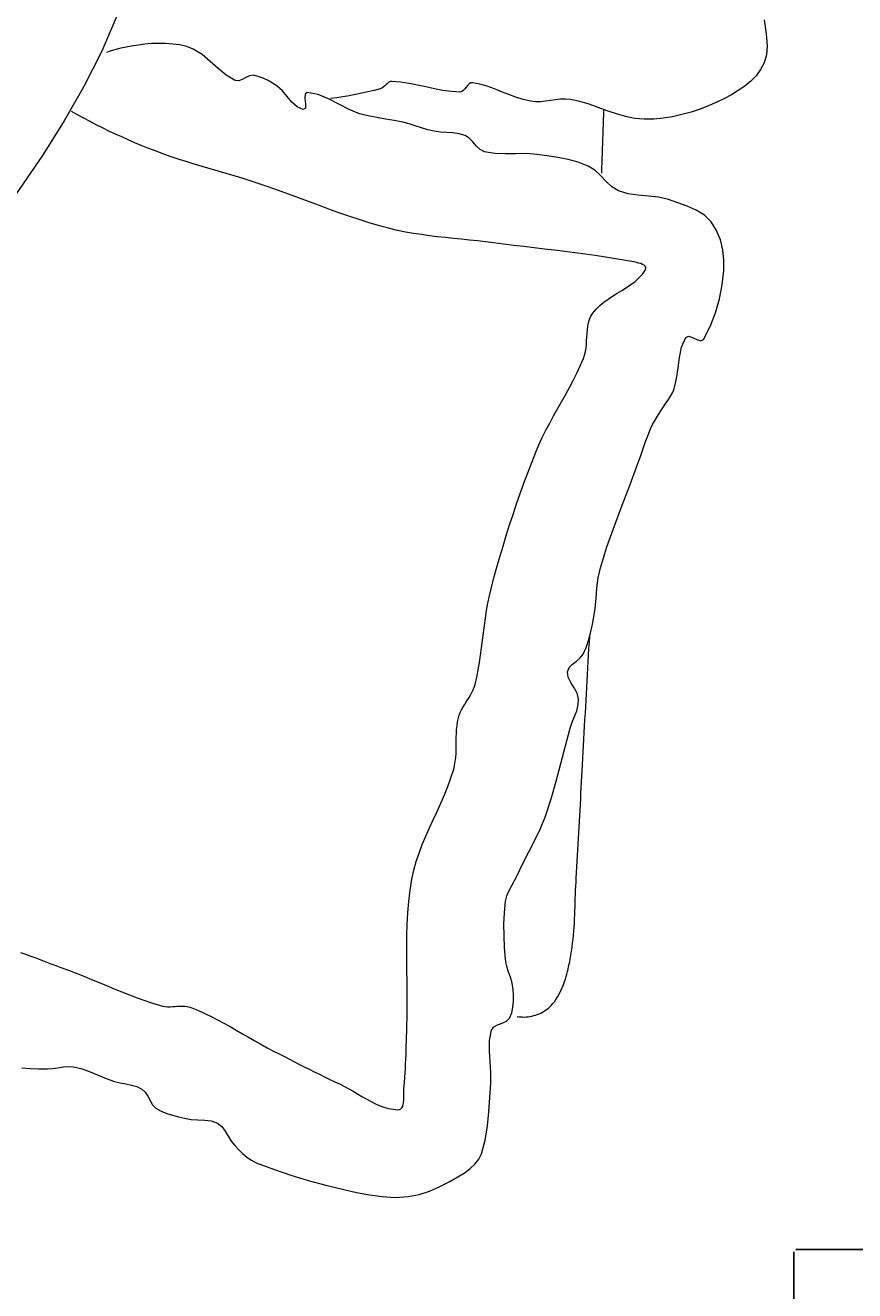
# Model space of a CAD drawing. Units: inches. Extents: x -15 to 423, y -713 to 71.
# Tile 21 of 24: x 340 to 364, y -173 to -137. Entities that reach past the tile are written whole.
import ezdxf

# ---------------------------------------------------------------- set-up
doc = ezdxf.new("R2010")
doc.units = ezdxf.units.IN
doc.header["$MEASUREMENT"] = 0
doc.layers.add('A-ANNO-DIMS', color=2, linetype='Continuous', lineweight=18)
doc.layers.add('A-FURN', color=9, linetype='Continuous', lineweight=13)
doc.styles.get("Standard").update_dxf_attribs({"font": 'arial.ttf'})
doc.dimstyles.get("Standard").update_dxf_attribs({"dimtxt": 0.18, "dimasz": 0.18, "dimexe": 0.18, "dimexo": 0.0625, "dimgap": 0.09, "dimtad": 0, "dimtih": 1, "dimtoh": 1, "dimdec": 0, "dimzin": 0, "dimdsep": 46, "dimlunit": 3, "dimtxsty": 'Standard', "dimcen": 0.09, "dimadec": 0, "dimazin": 0, "dimtfac": 1, "dimtdec": 0, "dimtofl": 0, "dimtmove": 0, "dimatfit": 3, "dimfxl": 1, "dimtolj": 1, "dimtzin": 0, "dimarcsym": 0})

# ---------------------------------------------------------------- blocks, each defined once
blk = doc.blocks.new('BED-DOUBLE')
for p, q in [((81.158, 34.884), (80.717, 33.859)), ((99.427, 34.751), (99.468, 34.498)), ((99.468, 34.498), (99.501, 34.248)), ((81.553, 34.002), (81.363, 33.968)), ((81.743, 34.034), (81.553, 34.002)), ((81.934, 34.06), (81.743, 34.034)), ((82.126, 34.077), (81.934, 34.06)), ((82.318, 34.081), (82.126, 34.077)), ((82.52, 34.075), (82.318, 34.081)), ((82.723, 34.063), (82.52, 34.075)), ((82.924, 34.037), (82.723, 34.063)), ((83.119, 33.992), (82.924, 34.037)), ((83.305, 33.921), (83.119, 33.992)), ((99.514, 34.001), (99.494, 33.761)), ((99.501, 34.248), (99.514, 34.001)), ((80.717, 33.859), (80.211, 32.862)), ((80.953, 33.862), (80.854, 33.825)), ((81.054, 33.894), (80.953, 33.862)), ((81.156, 33.923), (81.054, 33.894)), ((81.259, 33.948), (81.156, 33.923)), ((81.363, 33.968), (81.259, 33.948)), ((83.556, 33.766), (83.305, 33.921)), ((83.784, 33.574), (83.556, 33.766)), ((99.494, 33.761), (99.427, 33.528)), ((84.005, 33.372), (83.784, 33.574)), ((84.235, 33.184), (84.005, 33.372)), ((99.329, 33.34), (99.203, 33.169)), ((99.427, 33.528), (99.329, 33.34)), ((84.489, 33.037), (84.235, 33.184)), ((84.587, 33.027), (84.489, 33.037)), ((84.687, 33.064), (84.587, 33.027)), ((84.79, 33.12), (84.687, 33.064)), ((84.893, 33.168), (84.79, 33.12)), ((84.998, 33.18), (84.893, 33.168)), ((85.142, 33.148), (84.998, 33.18)), ((85.281, 33.097), (85.142, 33.148)), ((85.416, 33.031), (85.281, 33.097)), ((85.546, 32.954), (85.416, 33.031)), ((85.67, 32.872), (85.546, 32.954)), ((88.75, 32.919), (88.711, 32.883)), ((88.789, 32.953), (88.75, 32.919)), ((88.829, 32.982), (88.789, 32.953)), ((88.872, 33.001), (88.829, 32.982)), ((88.919, 33.007), (88.872, 33.001)), ((89.161, 32.986), (88.919, 33.007)), ((89.4, 32.95), (89.161, 32.986)), ((89.639, 32.903), (89.4, 32.95)), ((89.877, 32.851), (89.639, 32.903)), ((91.096, 32.937), (91.054, 32.895)), ((91.141, 32.965), (91.096, 32.937)), ((91.192, 32.971), (91.141, 32.965)), ((91.403, 32.931), (91.192, 32.971)), ((91.609, 32.871), (91.403, 32.931)), ((99.053, 33.014), (98.884, 32.874)), ((99.203, 33.169), (99.053, 33.014)), ((80.211, 32.862), (79.655, 31.89)), ((85.821, 32.738), (85.67, 32.872)), ((85.956, 32.578), (85.821, 32.738)), ((86.09, 32.42), (85.956, 32.578)), ((86.462, 32.647), (86.458, 32.521)), ((86.521, 32.696), (86.462, 32.647)), ((86.831, 32.634), (86.521, 32.696)), ((87.126, 32.514), (86.831, 32.634)), ((87.356, 32.547), (87.178, 32.524)), ((87.533, 32.573), (87.356, 32.547)), ((87.71, 32.603), (87.533, 32.573)), ((87.886, 32.636), (87.71, 32.603)), ((88.062, 32.672), (87.886, 32.636)), ((88.237, 32.712), (88.062, 32.672)), ((88.411, 32.755), (88.237, 32.712)), ((88.584, 32.801), (88.411, 32.755)), ((88.629, 32.82), (88.584, 32.801)), ((88.671, 32.849), (88.629, 32.82)), ((88.711, 32.883), (88.671, 32.849)), ((90.116, 32.799), (89.877, 32.851)), ((90.355, 32.755), (90.116, 32.799)), ((90.595, 32.722), (90.355, 32.755)), ((90.836, 32.707), (90.595, 32.722)), ((90.888, 32.719), (90.836, 32.707)), ((90.933, 32.75), (90.888, 32.719)), ((90.975, 32.795), (90.933, 32.75)), ((91.015, 32.845), (90.975, 32.795)), ((91.054, 32.895), (91.015, 32.845)), ((91.812, 32.797), (91.609, 32.871)), ((92.013, 32.716), (91.812, 32.797)), ((92.214, 32.634), (92.013, 32.716)), ((92.417, 32.558), (92.214, 32.634)), ((92.622, 32.492), (92.417, 32.558)), ((98.509, 32.632), (98.313, 32.528)), ((98.701, 32.747), (98.509, 32.632)), ((98.884, 32.874), (98.701, 32.747)), ((86.237, 32.289), (86.09, 32.42)), ((86.412, 32.213), (86.237, 32.289)), ((86.47, 32.251), (86.412, 32.213)), ((86.458, 32.521), (86.473, 32.372)), ((86.473, 32.372), (86.47, 32.251)), ((87.415, 32.365), (87.126, 32.514)), ((87.705, 32.216), (87.415, 32.365)), ((88.003, 32.096), (87.705, 32.216)), ((92.831, 32.445), (92.622, 32.492)), ((92.971, 32.431), (92.831, 32.445)), ((93.112, 32.434), (92.971, 32.431)), ((93.253, 32.448), (93.112, 32.434)), ((93.395, 32.468), (93.253, 32.448)), ((93.537, 32.488), (93.395, 32.468)), ((93.679, 32.503), (93.537, 32.488)), ((93.82, 32.507), (93.679, 32.503)), ((93.96, 32.495), (93.82, 32.507)), ((94.224, 32.44), (93.96, 32.495)), ((94.484, 32.363), (94.224, 32.44)), ((94.742, 32.273), (94.484, 32.363)), ((94.999, 32.179), (94.742, 32.273)), ((94.902, 32.129), (94.905, 32.22)), ((97.622, 32.227), (97.367, 32.141)), ((97.873, 32.324), (97.622, 32.227)), ((98.117, 32.433), (97.873, 32.324)), ((98.313, 32.528), (98.117, 32.433)), ((79.655, 31.89), (79.064, 30.944)), ((80.036, 32.061), (79.861, 32.158)), ((80.211, 31.966), (80.036, 32.061)), ((80.387, 31.873), (80.211, 31.966)), ((80.565, 31.782), (80.387, 31.873)), ((88.243, 32.032), (88.003, 32.096)), ((88.487, 31.984), (88.243, 32.032)), ((88.732, 31.944), (88.487, 31.984)), ((88.978, 31.903), (88.732, 31.944)), ((89.222, 31.853), (88.978, 31.903)), ((89.4, 31.805), (89.222, 31.853)), ((94.89, 31.768), (94.893, 31.858)), ((94.893, 31.858), (94.896, 31.949)), ((94.896, 31.949), (94.899, 32.039)), ((94.899, 32.039), (94.902, 32.129)), ((95.257, 32.09), (94.999, 32.179)), ((95.516, 32.015), (95.257, 32.09)), ((95.778, 31.962), (95.516, 32.015)), ((96.045, 31.939), (95.778, 31.962)), ((96.312, 31.945), (96.045, 31.939)), ((96.578, 31.969), (96.312, 31.945)), ((96.843, 32.011), (96.578, 31.969)), ((97.107, 32.069), (96.843, 32.011)), ((97.367, 32.141), (97.107, 32.069)), ((80.743, 31.692), (80.565, 31.782)), ((80.923, 31.605), (80.743, 31.692)), ((81.104, 31.52), (80.923, 31.605)), ((81.285, 31.437), (81.104, 31.52)), ((89.577, 31.751), (89.4, 31.805)), ((89.753, 31.695), (89.577, 31.751)), ((89.93, 31.642), (89.753, 31.695)), ((90.109, 31.598), (89.93, 31.642)), ((90.284, 31.573), (90.109, 31.598)), ((90.462, 31.562), (90.284, 31.573)), ((90.639, 31.551), (90.462, 31.562)), ((90.814, 31.528), (90.639, 31.551)), ((90.981, 31.479), (90.814, 31.528)), ((91.101, 31.403), (90.981, 31.479)), ((94.877, 31.407), (94.88, 31.497)), ((94.88, 31.497), (94.883, 31.587)), ((94.883, 31.587), (94.886, 31.678)), ((94.886, 31.678), (94.89, 31.768)), ((81.468, 31.355), (81.285, 31.437)), ((81.651, 31.276), (81.468, 31.355)), ((81.835, 31.199), (81.651, 31.276)), ((82.02, 31.124), (81.835, 31.199)), ((82.205, 31.052), (82.02, 31.124)), ((91.205, 31.296), (91.101, 31.403)), ((91.303, 31.181), (91.205, 31.296)), ((91.408, 31.082), (91.303, 31.181)), ((94.864, 31.046), (94.867, 31.136)), ((94.867, 31.136), (94.871, 31.226)), ((94.871, 31.226), (94.874, 31.317)), ((94.874, 31.317), (94.877, 31.407)), ((79.064, 30.944), (77.93, 29.295)), ((82.427, 30.969), (82.205, 31.052)), ((82.65, 30.89), (82.427, 30.969)), ((82.874, 30.815), (82.65, 30.89)), ((83.099, 30.743), (82.874, 30.815)), ((91.533, 31.019), (91.408, 31.082)), ((91.823, 30.969), (91.533, 31.019)), ((92.118, 30.958), (91.823, 30.969)), ((92.416, 30.963), (92.118, 30.958)), ((92.714, 30.966), (92.416, 30.963)), ((93.009, 30.944), (92.714, 30.966)), ((93.304, 30.904), (93.009, 30.944)), ((93.601, 30.858), (93.304, 30.904)), ((93.894, 30.8), (93.601, 30.858)), ((94.181, 30.722), (93.894, 30.8)), ((94.852, 30.684), (94.855, 30.775)), ((94.855, 30.775), (94.858, 30.865)), ((94.858, 30.865), (94.861, 30.955)), ((94.861, 30.955), (94.864, 31.046)), ((83.325, 30.673), (83.099, 30.743)), ((83.552, 30.605), (83.325, 30.673)), ((83.779, 30.538), (83.552, 30.605)), ((84.006, 30.471), (83.779, 30.538)), ((84.233, 30.404), (84.006, 30.471)), ((84.46, 30.337), (84.233, 30.404)), ((94.458, 30.617), (94.181, 30.722)), ((94.644, 30.5), (94.458, 30.617)), ((94.808, 30.347), (94.644, 30.5)), ((94.842, 30.414), (94.845, 30.504)), ((94.845, 30.504), (94.848, 30.594)), ((94.848, 30.594), (94.852, 30.684)), ((84.686, 30.269), (84.46, 30.337)), ((84.912, 30.198), (84.686, 30.269)), ((85.137, 30.125), (84.912, 30.198)), ((85.424, 30.028), (85.137, 30.125)), ((94.964, 30.181), (94.808, 30.347)), ((95.128, 30.029), (94.964, 30.181)), ((85.709, 29.927), (85.424, 30.028)), ((85.993, 29.823), (85.709, 29.927)), ((86.277, 29.718), (85.993, 29.823)), ((86.561, 29.612), (86.277, 29.718)), ((95.316, 29.916), (95.128, 30.029)), ((95.589, 29.834), (95.316, 29.916)), ((95.873, 29.793), (95.589, 29.834)), ((96.162, 29.768), (95.873, 29.793)), ((96.45, 29.735), (96.162, 29.768)), ((96.728, 29.668), (96.45, 29.735)), ((86.845, 29.506), (86.561, 29.612)), ((87.129, 29.401), (86.845, 29.506)), ((87.414, 29.298), (87.129, 29.401)), ((96.993, 29.581), (96.728, 29.668)), ((97.26, 29.486), (96.993, 29.581)), ((97.515, 29.372), (97.26, 29.486)), ((97.746, 29.225), (97.515, 29.372)), ((87.699, 29.198), (87.414, 29.298)), ((87.986, 29.102), (87.699, 29.198)), ((88.275, 29.012), (87.986, 29.102)), ((88.565, 28.927), (88.275, 29.012)), ((97.937, 29.036), (97.746, 29.225)), ((98.089, 28.796), (97.937, 29.036)), ((88.857, 28.849), (88.565, 28.927)), ((89.078, 28.797), (88.857, 28.849)), ((89.3, 28.752), (89.078, 28.797)), ((89.523, 28.712), (89.3, 28.752)), ((89.748, 28.678), (89.523, 28.712)), ((89.973, 28.647), (89.748, 28.678)), ((90.198, 28.62), (89.973, 28.647)), ((90.425, 28.595), (90.198, 28.62)), ((98.197, 28.529), (98.089, 28.796)), ((90.651, 28.572), (90.425, 28.595)), ((90.878, 28.549), (90.651, 28.572)), ((91.104, 28.526), (90.878, 28.549)), ((91.33, 28.502), (91.104, 28.526)), ((91.556, 28.476), (91.33, 28.502)), ((91.782, 28.447), (91.556, 28.476)), ((92.069, 28.41), (91.782, 28.447)), ((92.357, 28.373), (92.069, 28.41)), ((92.645, 28.338), (92.357, 28.373)), ((92.934, 28.304), (92.645, 28.338)), ((93.222, 28.269), (92.934, 28.304)), ((93.51, 28.235), (93.222, 28.269)), ((98.265, 28.245), (98.197, 28.529)), ((93.798, 28.2), (93.51, 28.235)), ((94.086, 28.163), (93.798, 28.2)), ((94.374, 28.125), (94.086, 28.163)), ((94.661, 28.085), (94.374, 28.125)), ((94.948, 28.043), (94.661, 28.085)), ((95.235, 27.997), (94.948, 28.043)), ((95.52, 27.948), (95.235, 27.997)), ((95.572, 27.94), (95.52, 27.948)), ((95.63, 27.93), (95.572, 27.94)), ((95.692, 27.919), (95.63, 27.93)), ((95.757, 27.907), (95.692, 27.919)), ((95.823, 27.892), (95.757, 27.907)), ((95.886, 27.876), (95.823, 27.892)), ((98.296, 27.954), (98.265, 28.245)), ((98.293, 27.667), (98.296, 27.954)), ((95.945, 27.858), (95.886, 27.876)), ((95.893, 27.455), (95.992, 27.563)), ((95.997, 27.836), (95.945, 27.858)), ((95.992, 27.563), (96.078, 27.682)), ((96.04, 27.812), (95.997, 27.836)), ((96.072, 27.785), (96.04, 27.812)), ((96.09, 27.755), (96.072, 27.785)), ((96.078, 27.682), (96.093, 27.72)), ((96.093, 27.72), (96.09, 27.755)), ((98.248, 27.261), (98.293, 27.667)), ((95.41, 27.101), (95.539, 27.183)), ((95.539, 27.183), (95.664, 27.267)), ((95.664, 27.267), (95.783, 27.357)), ((95.783, 27.357), (95.893, 27.455)), ((98.169, 26.859), (98.248, 27.261)), ((94.9, 26.77), (95.022, 26.858)), ((95.022, 26.858), (95.149, 26.941)), ((95.149, 26.941), (95.279, 27.022)), ((95.279, 27.022), (95.41, 27.101)), ((98.054, 26.464), (98.169, 26.859)), ((94.59, 26.455), (94.682, 26.57)), ((94.682, 26.57), (94.786, 26.674)), ((94.786, 26.674), (94.9, 26.77)), ((97.904, 26.082), (98.054, 26.464)), ((94.453, 26.088), (94.473, 26.186)), ((94.473, 26.186), (94.501, 26.28)), ((94.501, 26.28), (94.539, 26.37)), ((94.539, 26.37), (94.59, 26.455)), ((94.417, 25.678), (94.423, 25.782)), ((94.423, 25.782), (94.43, 25.886)), ((94.43, 25.886), (94.439, 25.988)), ((94.439, 25.988), (94.453, 26.088)), ((97.1, 25.5), (97.217, 25.769)), ((97.217, 25.769), (97.294, 25.805)), ((97.294, 25.805), (97.407, 25.772)), ((97.407, 25.772), (97.532, 25.714)), ((97.721, 25.718), (97.904, 26.082)), ((94.382, 25.372), (94.399, 25.472)), ((94.399, 25.472), (94.41, 25.575)), ((94.41, 25.575), (94.417, 25.678)), ((97.037, 25.21), (97.1, 25.5)), ((97.532, 25.714), (97.645, 25.681)), ((97.645, 25.681), (97.721, 25.718)), ((94.235, 24.969), (94.326, 25.179)), ((94.326, 25.179), (94.359, 25.273)), ((94.359, 25.273), (94.382, 25.372)), ((96.999, 24.911), (97.037, 25.21)), ((94.035, 24.558), (94.138, 24.762)), ((94.138, 24.762), (94.235, 24.969)), ((96.959, 24.61), (96.999, 24.911)), ((93.818, 24.155), (93.928, 24.356)), ((93.928, 24.356), (94.035, 24.558)), ((96.841, 24.205), (96.89, 24.32)), ((96.89, 24.32), (96.959, 24.61)), ((93.706, 23.955), (93.818, 24.155)), ((96.634, 23.889), (96.707, 23.993)), ((96.707, 23.993), (96.778, 24.097)), ((96.778, 24.097), (96.841, 24.205)), ((93.482, 23.555), (93.593, 23.755)), ((93.593, 23.755), (93.706, 23.955)), ((96.421, 23.549), (96.494, 23.666)), ((96.494, 23.666), (96.566, 23.783)), ((96.566, 23.783), (96.634, 23.889)), ((93.265, 23.152), (93.372, 23.354)), ((93.372, 23.354), (93.482, 23.555)), ((96.221, 23.189), (96.281, 23.312)), ((96.281, 23.312), (96.349, 23.432)), ((96.349, 23.432), (96.421, 23.549)), ((93.068, 22.74), (93.164, 22.947)), ((93.164, 22.947), (93.265, 23.152)), ((96.069, 22.8), (96.141, 22.996)), ((96.141, 22.996), (96.221, 23.189)), ((92.864, 22.239), (92.979, 22.53)), ((92.979, 22.53), (93.068, 22.74)), ((95.935, 22.404), (96.002, 22.602)), ((96.002, 22.602), (96.069, 22.8)), ((92.753, 21.948), (92.864, 22.239)), ((95.648, 21.619), (95.867, 22.207)), ((95.867, 22.207), (95.935, 22.404)), ((92.644, 21.655), (92.753, 21.948)), ((92.539, 21.361), (92.644, 21.655)), ((95.422, 21.034), (95.648, 21.619)), ((92.436, 21.066), (92.539, 21.361)), ((92.24, 20.473), (92.337, 20.77)), ((92.337, 20.77), (92.436, 21.066)), ((95.2, 20.447), (95.422, 21.034)), ((92.146, 20.175), (92.24, 20.473)), ((94.99, 19.857), (95.2, 20.447)), ((92.055, 19.876), (92.146, 20.175)), ((91.967, 19.576), (92.055, 19.876)), ((94.804, 19.259), (94.99, 19.857)), ((91.882, 19.276), (91.967, 19.576)), ((91.719, 18.673), (91.799, 18.975)), ((91.799, 18.975), (91.882, 19.276)), ((94.707, 18.69), (94.742, 18.977)), ((94.742, 18.977), (94.804, 19.259)), ((91.669, 18.468), (91.719, 18.673)), ((94.683, 18.401), (94.707, 18.69)), ((91.59, 18.053), (91.627, 18.261)), ((91.627, 18.261), (91.669, 18.468)), ((94.657, 18.111), (94.683, 18.401)), ((91.558, 17.844), (91.59, 18.053)), ((94.613, 17.825), (94.657, 18.111)), ((91.502, 17.424), (91.529, 17.634)), ((91.529, 17.634), (91.558, 17.844)), ((94.524, 17.415), (94.571, 17.62)), ((94.571, 17.62), (94.613, 17.825)), ((91.449, 17.004), (91.476, 17.214)), ((91.476, 17.214), (91.502, 17.424)), ((94.4, 17.014), (94.468, 17.212)), ((94.468, 17.212), (94.524, 17.415)), ((94.494, 17.16), (94.504, 17.342)), ((91.421, 16.794), (91.449, 17.004)), ((94.236, 16.716), (94.317, 16.822)), ((94.317, 16.822), (94.4, 17.014)), ((94.473, 16.795), (94.483, 16.977)), ((94.483, 16.977), (94.494, 17.16)), ((91.353, 16.376), (91.389, 16.585)), ((91.389, 16.585), (91.421, 16.794)), ((93.922, 16.444), (94.013, 16.539)), ((94.013, 16.539), (94.126, 16.626)), ((94.126, 16.626), (94.236, 16.716)), ((94.452, 16.43), (94.463, 16.612)), ((94.463, 16.612), (94.473, 16.795)), ((91.264, 15.963), (91.312, 16.169)), ((91.312, 16.169), (91.353, 16.376)), ((93.877, 16.327), (93.922, 16.444)), ((93.898, 16.169), (93.877, 16.327)), ((93.971, 16.019), (93.898, 16.169)), ((94.432, 16.065), (94.442, 16.248)), ((94.442, 16.248), (94.452, 16.43)), ((91.137, 15.668), (91.176, 15.739)), ((91.176, 15.739), (91.211, 15.812)), ((91.211, 15.812), (91.241, 15.886)), ((91.241, 15.886), (91.264, 15.963)), ((94.065, 15.871), (93.971, 16.019)), ((94.149, 15.721), (94.065, 15.871)), ((94.411, 15.7), (94.421, 15.883)), ((94.421, 15.883), (94.432, 16.065)), ((90.921, 15.319), (90.963, 15.389)), ((90.963, 15.389), (91.007, 15.458)), ((91.007, 15.458), (91.051, 15.528)), ((91.051, 15.528), (91.095, 15.597)), ((91.095, 15.597), (91.137, 15.668)), ((94.135, 15.225), (94.177, 15.392)), ((94.189, 15.562), (94.149, 15.721)), ((94.177, 15.392), (94.189, 15.562)), ((94.391, 15.335), (94.401, 15.518)), ((94.401, 15.518), (94.411, 15.7)), ((90.771, 14.913), (90.794, 15.023)), ((90.794, 15.023), (90.817, 15.1)), ((90.817, 15.1), (90.847, 15.175)), ((90.847, 15.175), (90.882, 15.247)), ((90.882, 15.247), (90.921, 15.319)), ((94.01, 14.897), (94.075, 15.061)), ((94.075, 15.061), (94.135, 15.225)), ((94.37, 14.971), (94.38, 15.153)), ((94.38, 15.153), (94.391, 15.335)), ((90.738, 14.577), (90.744, 14.69)), ((90.744, 14.69), (90.755, 14.802)), ((90.755, 14.802), (90.771, 14.913)), ((93.82, 14.232), (93.955, 14.732)), ((93.955, 14.732), (94.01, 14.897)), ((94.35, 14.606), (94.36, 14.788)), ((94.36, 14.788), (94.37, 14.971)), ((90.734, 14.351), (90.735, 14.464)), ((90.734, 14.237), (90.734, 14.351)), ((90.735, 14.464), (90.738, 14.577)), ((94.329, 14.241), (94.34, 14.423)), ((94.34, 14.423), (94.35, 14.606)), ((90.72, 13.898), (90.728, 14.011)), ((90.728, 14.011), (90.732, 14.124)), ((90.732, 14.124), (90.734, 14.237)), ((93.691, 13.73), (93.82, 14.232)), ((94.309, 13.876), (94.319, 14.058)), ((94.319, 14.058), (94.329, 14.241)), ((90.662, 13.568), (90.688, 13.677)), ((90.688, 13.677), (90.707, 13.787)), ((90.707, 13.787), (90.72, 13.898)), ((93.559, 13.23), (93.691, 13.73)), ((94.29, 13.533), (94.299, 13.693)), ((94.299, 13.693), (94.309, 13.876)), ((90.497, 13.085), (90.584, 13.325)), ((90.584, 13.325), (90.662, 13.568)), ((94.273, 13.213), (94.281, 13.373)), ((94.281, 13.373), (94.29, 13.533)), ((90.4, 12.848), (90.497, 13.085)), ((93.416, 12.733), (93.559, 13.23)), ((94.248, 12.733), (94.256, 12.893)), ((94.256, 12.893), (94.264, 13.053)), ((94.264, 13.053), (94.273, 13.213)), ((90.191, 12.378), (90.297, 12.612)), ((90.297, 12.612), (90.4, 12.848)), ((93.253, 12.242), (93.416, 12.733)), ((94.231, 12.412), (94.239, 12.572)), ((94.239, 12.572), (94.248, 12.733)), ((90.083, 12.145), (90.191, 12.378)), ((93.115, 11.899), (93.253, 12.242)), ((94.214, 12.092), (94.223, 12.252)), ((94.223, 12.252), (94.231, 12.412)), ((89.871, 11.676), (89.975, 11.911)), ((89.975, 11.911), (90.083, 12.145)), ((92.957, 11.564), (93.115, 11.899)), ((94.197, 11.772), (94.206, 11.932)), ((94.206, 11.932), (94.214, 12.092)), ((89.772, 11.441), (89.871, 11.676)), ((92.788, 11.233), (92.957, 11.564)), ((94.171, 11.291), (94.18, 11.451)), ((94.18, 11.451), (94.189, 11.612)), ((94.189, 11.612), (94.197, 11.772)), ((89.6, 10.961), (89.681, 11.202)), ((89.681, 11.202), (89.772, 11.441)), ((92.618, 10.903), (92.788, 11.233)), ((94.153, 10.971), (94.162, 11.131)), ((94.162, 11.131), (94.171, 11.291)), ((89.532, 10.717), (89.6, 10.961)), ((92.454, 10.571), (92.618, 10.903)), ((94.134, 10.651), (94.143, 10.811)), ((94.143, 10.811), (94.153, 10.971)), ((89.428, 10.15), (89.478, 10.468)), ((89.478, 10.468), (89.532, 10.717)), ((92.3, 10.285), (92.38, 10.427)), ((92.38, 10.427), (92.454, 10.571)), ((94.111, 10.262), (94.117, 10.376)), ((94.117, 10.376), (94.124, 10.491)), ((94.124, 10.491), (94.134, 10.651)), ((89.39, 9.83), (89.428, 10.15)), ((92.163, 9.994), (92.224, 10.142)), ((92.224, 10.142), (92.3, 10.285)), ((94.097, 9.917), (94.101, 10.032)), ((94.101, 10.032), (94.106, 10.147)), ((94.106, 10.147), (94.111, 10.262)), ((89.363, 9.509), (89.39, 9.83)), ((92.092, 9.515), (92.125, 9.84)), ((92.125, 9.84), (92.163, 9.994)), ((94.085, 9.572), (94.089, 9.687)), ((94.089, 9.687), (94.093, 9.802)), ((94.093, 9.802), (94.097, 9.917)), ((89.346, 9.187), (89.363, 9.509)), ((92.079, 9.189), (92.092, 9.515)), ((94.069, 9.227), (94.075, 9.342)), ((94.075, 9.342), (94.08, 9.457)), ((94.08, 9.457), (94.085, 9.572)), ((89.337, 8.864), (89.346, 9.187)), ((92.083, 8.861), (92.079, 9.189)), ((94.045, 8.883), (94.054, 8.997)), ((94.054, 8.997), (94.062, 9.112)), ((94.062, 9.112), (94.069, 9.227)), ((89.334, 8.541), (89.337, 8.864)), ((92.1, 8.534), (92.083, 8.861)), ((94.007, 8.541), (94.021, 8.655)), ((94.021, 8.655), (94.034, 8.769)), ((94.034, 8.769), (94.045, 8.883)), ((78.425, 8.391), (78.568, 8.342)), ((78.568, 8.342), (78.711, 8.291)), ((78.711, 8.291), (78.854, 8.238)), ((78.854, 8.238), (78.996, 8.184)), ((89.335, 8.217), (89.334, 8.541)), ((92.125, 8.207), (92.1, 8.534)), ((93.951, 8.202), (93.972, 8.315)), ((93.972, 8.315), (93.991, 8.428)), ((93.991, 8.428), (94.007, 8.541)), ((78.996, 8.184), (79.138, 8.129)), ((79.138, 8.129), (79.28, 8.075)), ((79.28, 8.075), (79.422, 8.021)), ((79.422, 8.021), (79.564, 7.969)), ((79.564, 7.969), (79.781, 7.889)), ((79.781, 7.889), (79.997, 7.806)), ((89.338, 7.893), (89.335, 8.217)), ((89.343, 7.568), (89.338, 7.893)), ((92.154, 8.033), (92.125, 8.207)), ((92.204, 7.862), (92.154, 8.033)), ((93.874, 7.851), (93.891, 7.921)), ((93.891, 7.921), (93.907, 7.992)), ((93.907, 7.992), (93.923, 8.062)), ((93.923, 8.062), (93.937, 8.132)), ((93.937, 8.132), (93.951, 8.202)), ((79.997, 7.806), (80.213, 7.72)), ((80.213, 7.72), (80.428, 7.633)), ((80.428, 7.633), (80.642, 7.545)), ((80.642, 7.545), (80.857, 7.457)), ((89.347, 7.244), (89.343, 7.568)), ((92.261, 7.693), (92.204, 7.862)), ((92.309, 7.522), (92.261, 7.693)), ((92.337, 7.347), (92.309, 7.522)), ((93.769, 7.504), (93.793, 7.572)), ((93.793, 7.572), (93.815, 7.641)), ((93.815, 7.641), (93.836, 7.711)), ((93.836, 7.711), (93.856, 7.781)), ((93.856, 7.781), (93.874, 7.851)), ((80.857, 7.457), (81.071, 7.369)), ((81.071, 7.369), (81.286, 7.282)), ((81.286, 7.282), (81.502, 7.197)), ((81.502, 7.197), (81.718, 7.115)), ((89.349, 6.92), (89.347, 7.244)), ((92.346, 7.181), (92.337, 7.347)), ((92.348, 7.012), (92.346, 7.181)), ((93.584, 7.118), (93.62, 7.179)), ((93.62, 7.179), (93.654, 7.241)), ((93.654, 7.241), (93.686, 7.305)), ((93.686, 7.305), (93.715, 7.37)), ((93.715, 7.37), (93.743, 7.436)), ((93.743, 7.436), (93.769, 7.504)), ((81.718, 7.115), (81.936, 7.036)), ((81.936, 7.036), (82.155, 6.961)), ((82.155, 6.961), (82.375, 6.89)), ((82.375, 6.89), (82.442, 6.874)), ((82.442, 6.874), (82.51, 6.864)), ((82.51, 6.864), (82.579, 6.86)), ((82.579, 6.86), (82.648, 6.859)), ((82.648, 6.859), (82.719, 6.862)), ((82.719, 6.862), (82.789, 6.866)), ((82.789, 6.866), (82.86, 6.871)), ((82.86, 6.871), (82.93, 6.874)), ((82.93, 6.874), (83, 6.875)), ((83, 6.875), (83.069, 6.872)), ((83.069, 6.872), (83.136, 6.865)), ((83.136, 6.865), (83.203, 6.851)), ((83.203, 6.851), (83.268, 6.829)), ((83.268, 6.829), (83.452, 6.752)), ((89.346, 6.597), (89.349, 6.92)), ((92.3, 6.684), (92.334, 6.846)), ((92.334, 6.846), (92.348, 7.012)), ((93.301, 6.791), (93.341, 6.823)), ((93.341, 6.823), (93.379, 6.857)), ((93.379, 6.857), (93.414, 6.893)), ((93.414, 6.893), (93.461, 6.946)), ((93.461, 6.946), (93.505, 7.002)), ((93.505, 7.002), (93.546, 7.059)), ((93.546, 7.059), (93.584, 7.118)), ((83.452, 6.752), (83.634, 6.669)), ((83.634, 6.669), (83.814, 6.581)), ((83.814, 6.581), (83.992, 6.489)), ((83.992, 6.489), (84.169, 6.394)), ((89.337, 6.274), (89.346, 6.597)), ((92.034, 6.393), (92.155, 6.448)), ((92.155, 6.448), (92.239, 6.533)), ((92.239, 6.533), (92.3, 6.684)), ((92.454, 6.586), (92.504, 6.578)), ((92.504, 6.578), (92.555, 6.572)), ((92.555, 6.572), (92.606, 6.569)), ((92.606, 6.569), (92.659, 6.568)), ((92.659, 6.568), (92.711, 6.571)), ((92.711, 6.571), (92.764, 6.576)), ((92.764, 6.576), (92.816, 6.584)), ((92.816, 6.584), (92.869, 6.594)), ((92.869, 6.594), (92.921, 6.607)), ((92.921, 6.607), (92.972, 6.622)), ((92.972, 6.622), (93.023, 6.639)), ((93.023, 6.639), (93.072, 6.659)), ((93.072, 6.659), (93.121, 6.681)), ((93.121, 6.681), (93.168, 6.706)), ((93.168, 6.706), (93.214, 6.732)), ((93.214, 6.732), (93.258, 6.76)), ((93.258, 6.76), (93.301, 6.791)), ((84.169, 6.394), (84.344, 6.296)), ((84.344, 6.296), (84.519, 6.197)), ((84.519, 6.197), (84.693, 6.097)), ((84.693, 6.097), (84.867, 5.996)), ((89.329, 6.016), (89.333, 6.145)), ((89.333, 6.145), (89.337, 6.274)), ((91.675, 5.904), (91.726, 6.196)), ((91.726, 6.196), (91.792, 6.289)), ((91.792, 6.289), (91.903, 6.348)), ((91.903, 6.348), (92.034, 6.393)), ((84.867, 5.996), (85.042, 5.896)), ((85.042, 5.896), (85.217, 5.798)), ((85.217, 5.798), (85.393, 5.701)), ((89.318, 5.631), (89.322, 5.759)), ((89.322, 5.759), (89.325, 5.888)), ((89.325, 5.888), (89.329, 6.016)), ((91.671, 5.606), (91.675, 5.904)), ((85.393, 5.701), (85.57, 5.607)), ((85.57, 5.607), (85.714, 5.533)), ((85.714, 5.533), (85.858, 5.459)), ((85.858, 5.459), (86.002, 5.385)), ((86.002, 5.385), (86.146, 5.312)), ((89.304, 5.245), (89.31, 5.374)), ((89.31, 5.374), (89.314, 5.502)), ((89.314, 5.502), (89.318, 5.631)), ((91.692, 5.303), (91.671, 5.606)), ((78.457, 5.132), (78.699, 5.116)), ((78.699, 5.116), (78.941, 5.108)), ((78.941, 5.108), (79.183, 5.102)), ((79.183, 5.102), (79.332, 5.11)), ((79.332, 5.11), (79.48, 5.134)), ((79.48, 5.134), (79.629, 5.159)), ((79.629, 5.159), (79.777, 5.173)), ((79.777, 5.173), (79.923, 5.162)), ((79.923, 5.162), (80.161, 5.102)), ((80.161, 5.102), (80.392, 5.019)), ((80.392, 5.019), (80.62, 4.925)), ((86.146, 5.312), (86.29, 5.238)), ((86.29, 5.238), (86.435, 5.165)), ((86.435, 5.165), (86.579, 5.093)), ((86.579, 5.093), (86.724, 5.021)), ((86.724, 5.021), (86.869, 4.949)), ((89.29, 4.988), (89.298, 5.117)), ((89.298, 5.117), (89.304, 5.245)), ((91.713, 5), (91.692, 5.303)), ((80.62, 4.925), (80.848, 4.83)), ((80.848, 4.83), (81.079, 4.745)), ((81.079, 4.745), (81.235, 4.705)), ((81.235, 4.705), (81.396, 4.676)), ((81.396, 4.676), (81.555, 4.645)), ((86.869, 4.949), (87.014, 4.878)), ((87.014, 4.878), (87.16, 4.807)), ((87.16, 4.807), (87.306, 4.737)), ((87.306, 4.737), (87.452, 4.667)), ((87.452, 4.667), (87.575, 4.606)), ((89.258, 4.604), (89.27, 4.732)), ((89.27, 4.732), (89.281, 4.86)), ((89.281, 4.86), (89.29, 4.988)), ((91.681, 4.297), (91.709, 4.7)), ((91.709, 4.7), (91.713, 5)), ((81.555, 4.645), (81.709, 4.601)), ((81.709, 4.601), (81.851, 4.532)), ((81.851, 4.532), (81.946, 4.442)), ((81.946, 4.442), (82.018, 4.328)), ((82.018, 4.328), (82.082, 4.205)), ((87.575, 4.606), (87.698, 4.539)), ((87.698, 4.539), (87.82, 4.469)), ((87.82, 4.469), (87.942, 4.397)), ((87.942, 4.397), (88.064, 4.325)), ((88.064, 4.325), (88.186, 4.254)), ((89.252, 4.487), (89.254, 4.549)), ((89.252, 4.422), (89.252, 4.487)), ((89.253, 4.355), (89.252, 4.422)), ((89.252, 4.287), (89.253, 4.355)), ((89.254, 4.549), (89.258, 4.604)), ((91.655, 3.892), (91.681, 4.297)), ((82.082, 4.205), (82.153, 4.09)), ((82.153, 4.09), (82.246, 3.997)), ((82.246, 3.997), (82.395, 3.911)), ((88.186, 4.254), (88.309, 4.187)), ((88.309, 4.187), (88.434, 4.125)), ((88.434, 4.125), (88.56, 4.069)), ((88.56, 4.069), (88.688, 4.022)), ((88.688, 4.022), (88.818, 3.985)), ((88.818, 3.985), (88.951, 3.96)), ((88.951, 3.96), (89.086, 3.947)), ((89.086, 3.947), (89.133, 3.953)), ((89.133, 3.953), (89.17, 3.973)), ((89.17, 3.973), (89.199, 4.005)), ((89.199, 4.005), (89.22, 4.048)), ((89.22, 4.048), (89.235, 4.099)), ((89.235, 4.099), (89.244, 4.157)), ((89.244, 4.157), (89.25, 4.221)), ((89.25, 4.221), (89.252, 4.287)), ((82.395, 3.911), (82.553, 3.845)), ((82.553, 3.845), (82.719, 3.791)), ((82.719, 3.791), (82.887, 3.747)), ((82.887, 3.747), (83.056, 3.706)), ((83.056, 3.706), (83.243, 3.677)), ((83.243, 3.677), (83.435, 3.667)), ((83.435, 3.667), (83.627, 3.658)), ((83.627, 3.658), (83.812, 3.631)), ((83.812, 3.631), (83.985, 3.566)), ((91.616, 3.489), (91.655, 3.892)), ((83.985, 3.566), (84.108, 3.47)), ((84.108, 3.47), (84.205, 3.343)), ((84.205, 3.343), (84.289, 3.201)), ((91.551, 3.092), (91.616, 3.489)), ((84.289, 3.201), (84.374, 3.059)), ((84.374, 3.059), (84.475, 2.933)), ((84.475, 2.933), (84.585, 2.821)), ((91.446, 2.705), (91.551, 3.092)), ((84.585, 2.821), (84.699, 2.711)), ((84.699, 2.711), (84.819, 2.609)), ((84.819, 2.609), (84.947, 2.521)), ((84.947, 2.521), (85.085, 2.451)), ((91.262, 2.407), (91.371, 2.547)), ((91.371, 2.547), (91.446, 2.705)), ((85.085, 2.451), (85.568, 2.267)), ((85.568, 2.267), (86.057, 2.099)), ((90.829, 2.078), (90.981, 2.174)), ((90.981, 2.174), (91.129, 2.283)), ((91.129, 2.283), (91.262, 2.407)), ((86.057, 2.099), (86.552, 1.947)), ((86.552, 1.947), (87.051, 1.812)), ((87.051, 1.812), (87.554, 1.691)), ((90.272, 1.775), (90.554, 1.922)), ((90.554, 1.922), (90.829, 2.078)), ((87.554, 1.691), (87.914, 1.613)), ((87.914, 1.613), (88.278, 1.543)), ((88.278, 1.543), (88.645, 1.493)), ((88.645, 1.493), (89.011, 1.472)), ((89.011, 1.472), (89.376, 1.492)), ((89.376, 1.492), (89.683, 1.551)), ((89.683, 1.551), (89.982, 1.649)), ((89.982, 1.649), (90.272, 1.775))]:
    blk.add_line(p, q)
blk = doc.blocks.new('*D31')
at = {"layer": 'A-ANNO-DIMS', "color": 0, "lineweight": -2, "transparency": 16777216}
for p, q in [((261.638, -171.991), (261.638, -187.148)), ((361.906, -171.991), (361.906, -187.148)), ((261.818, -186.968), (310.634, -186.968)), ((361.726, -186.968), (312.91, -186.968))]:
    blk.add_line(p, q, dxfattribs=at)
at = {"layer": 'A-ANNO-DIMS', "color": 0, "transparency": 16777216}
for points in [[(261.818, -186.938), (261.818, -186.998), (261.638, -186.968)], [(361.726, -186.938), (361.726, -186.998), (361.906, -186.968)]]:
    blk.add_solid(points, dxfattribs=at)
at = {"layer": 'Defpoints', "color": 0, "transparency": 16777216}
for p in [(261.638, -171.928), (361.906, -171.928), (361.906, -186.968)]:
    blk.add_point(p, dxfattribs=at)
at = {"layer": 'A-ANNO-DIMS', "color": 0, "transparency": 16777216, "insert": (311.772, -186.968), "char_height": 0.18, "attachment_point": 5}
blk.add_mtext('\\A1;BED 8\'-4 1/2" TYP.', dxfattribs=at)
blk = doc.blocks.new('*D32')
at = {"layer": 'A-ANNO-DIMS', "color": 0, "lineweight": -2, "transparency": 16777216}
for p, q in [((361.968, -101.283), (377.126, -101.283)), ((376.946, -101.463), (376.946, -136.422)), ((376.946, -171.748), (376.946, -136.788)), ((361.968, -171.928), (377.126, -171.928))]:
    blk.add_line(p, q, dxfattribs=at)
at = {"layer": 'A-ANNO-DIMS', "color": 0, "transparency": 16777216}
for points in [[(376.916, -101.463), (376.976, -101.463), (376.946, -101.283)], [(376.916, -171.748), (376.976, -171.748), (376.946, -171.928)]]:
    blk.add_solid(points, dxfattribs=at)
at = {"layer": 'Defpoints', "color": 0, "transparency": 16777216}
for p in [(361.906, -101.283), (376.946, -101.283), (361.906, -171.928)]:
    blk.add_point(p, dxfattribs=at)
at = {"layer": 'A-ANNO-DIMS', "color": 0, "transparency": 16777216, "insert": (376.946, -136.605), "char_height": 0.18, "attachment_point": 5}
blk.add_mtext('\\A1;5\'-10 1/2" TYP.', dxfattribs=at)

msp = doc.modelspace()

# ---------------------------------------------------------------- block references
at = {"layer": 'A-FURN'}
msp.add_blockref('BED-DOUBLE', (261.638, -171.928), dxfattribs=at)

# ---------------------------------------------------------------- dimensions: what is measured, and where the dimension line sits
at = {"layer": 'A-ANNO-DIMS'}
dim = msp.add_linear_dim(base=(376.946, -101.283), p1=(361.906, -171.928), p2=(361.906, -101.283), angle=90, text='<> TYP.', dimstyle='Standard', override={"dimdec": 1, "dimlfac": 1, "dimrnd": 0, "dimzin": 1, "dimdsep": 46, "dimlunit": 4, "dimfrac": 2}, dxfattribs=at)
dim.commit()
dim.dimension.update_dxf_attribs({"geometry": '*D32', "text_midpoint": (376.946, -136.605)})
dim = msp.add_linear_dim(base=(361.906, -186.968), p1=(261.638, -171.928), p2=(361.906, -171.928), text='BED <> TYP.', dimstyle='Standard', override={"dimdec": 1, "dimlfac": 1, "dimrnd": 0, "dimzin": 1, "dimdsep": 46, "dimlunit": 4, "dimfrac": 2}, dxfattribs=at)
dim.commit()
dim.dimension.update_dxf_attribs({"geometry": '*D31', "text_midpoint": (311.772, -186.968)})

doc.saveas('drawing.dxf')
